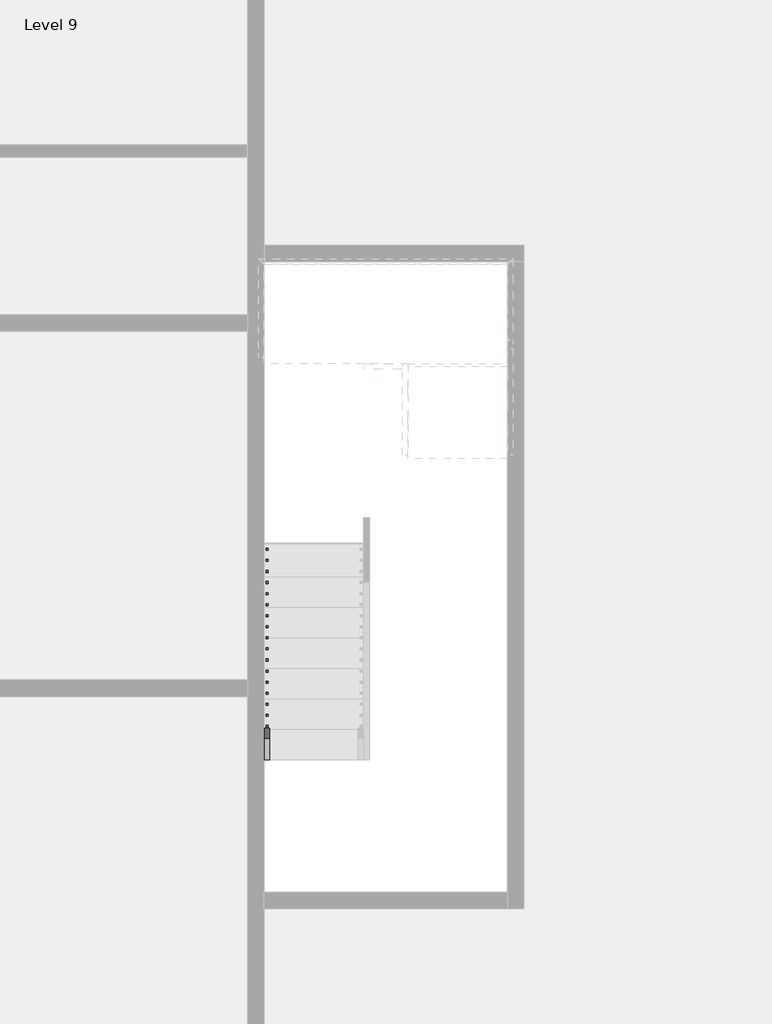
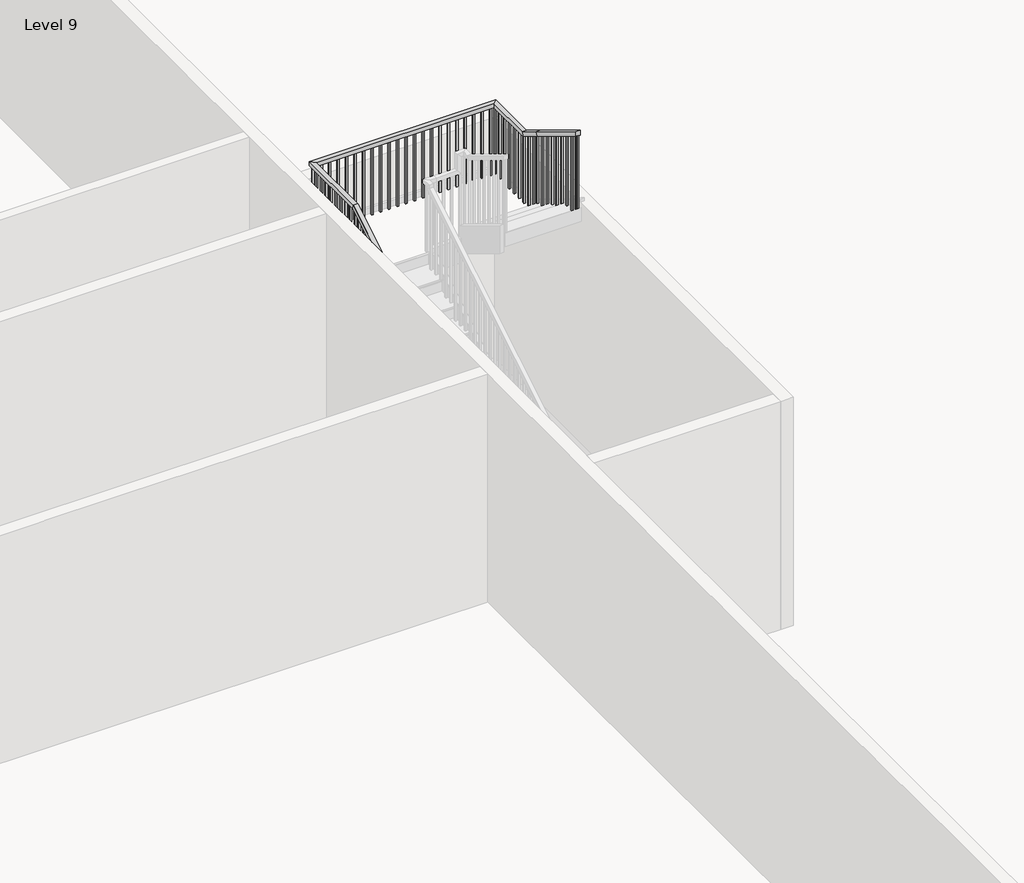
# One storey, part 6 of 8: 1 railing.
"""IFC4 building model written with IfcOpenShell, lengths in millimetres."""

from ifc_helpers import new_model, si_unit, frame, origin, place, context, project, spatial, polyline, outline, extrude, faceted_brep, element, save

model = new_model("IFC4")

# Units and contexts
model_context = context("Model", 3, world=origin())
ifc_project = project(units=[si_unit("LENGTHUNIT", "METRE", prefix="MILLI")], contexts=[model_context])

# Site, building, storey
site = spatial("IfcSite", under=ifc_project)
building = spatial("IfcBuilding", under=site)
storey = spatial("IfcBuildingStorey", under=building, Name="Level 9", Elevation=49618.6172466)

# Railing
placement = place(None, origin())
element("IfcRailing", 1, ObjectType="Handrail - Rectangular", at=placement, inside=storey, context=model_context, shape_type="SolidModel", body=[
    faceted_brep([(-3617.4415084, -23154.3851539, 50702.3505799), (-3617.4415084, -23154.3851539, 50642.9491197), (-3566.6415084, -23154.3851539, 50642.9491197), (-3566.6415084, -23154.3851539, 50702.3505799), (-3617.4415084, -19522.1851539, 52903.6839133), (-3617.4415084, -19507.9927445, 52852.8839133), (-3566.6415084, -19507.9927445, 52852.8839133), (-3566.6415084, -19522.1851539, 52903.6839133), (-3617.4415084, -18607.7851539, 52903.6839133), (-3617.4415084, -18607.7851539, 52852.8839133), (-3566.6415084, -18658.5851539, 52852.8839133), (-3566.6415084, -18658.5851539, 52903.6839133), (-1382.2415084, -18607.7851539, 52903.6839133), (-1382.2415084, -18607.7851539, 52852.8839133), (-1433.0415084, -18658.5851539, 52852.8839133), (-1433.0415084, -18658.5851539, 52903.6839133), (-1382.2415084, -19242.7851539, 52903.6839133), (-1382.2415084, -19256.9775633, 52852.8839133), (-1433.0415084, -19256.9775633, 52852.8839133), (-1433.0415084, -19242.7851539, 52903.6839133), (-1382.2415084, -19522.1851539, 53073.0172466), (-1382.2415084, -19548.5148811, 53029.5731968), (-1433.0415084, -19548.5148811, 53029.5731968), (-1433.0415084, -19522.1851539, 53073.0172466), (-1382.2415084, -20360.3851539, 53581.0172466), (-1433.0415084, -20360.3851539, 53581.0172466), (-1433.0415084, -20360.3851539, 53521.6157863), (-1382.2415084, -20360.3851539, 53521.6157863)], [[[0, 1, 2, 3]], [[1, 0, 4, 5]], [[2, 1, 5, 6]], [[3, 2, 6, 7]], [[0, 3, 7, 4]], [[5, 4, 8, 9]], [[6, 5, 9, 10]], [[7, 6, 10, 11]], [[4, 7, 11, 8]], [[9, 8, 12, 13]], [[10, 9, 13, 14]], [[11, 10, 14, 15]], [[8, 11, 15, 12]], [[13, 12, 16, 17]], [[14, 13, 17, 18]], [[15, 14, 18, 19]], [[12, 15, 19, 16]], [[17, 16, 20, 21]], [[18, 17, 21, 22]], [[19, 18, 22, 23]], [[16, 19, 23, 20]], [[24, 25, 26, 27]], [[21, 20, 24, 27]], [[22, 21, 27, 26]], [[23, 22, 26, 25]], [[20, 23, 25, 24]]]),
    extrude(outline(polyline([(-20325.4601539, 53500.4491197), (-20325.4601539, 52497.2839133), (-20344.5101539, 52497.2839133), (-20344.5101539, 53511.9945742), (-20325.4601539, 53500.4491197)])), frame((-1417.1665084, 0.0, 0.0), z_axis=(1.0, 0.0, 0.0), x_axis=(0.0, 1.0, 0.0)), (0.0, 0.0, 1.0), 19.05),
    extrude(outline(polyline([(-20223.8601539, 53438.8733621), (-20223.8601539, 52497.2839133), (-20242.9101539, 52497.2839133), (-20242.9101539, 53450.4188166), (-20223.8601539, 53438.8733621)])), frame((-1417.1665084, 0.0, 0.0), z_axis=(1.0, 0.0, 0.0), x_axis=(0.0, 1.0, 0.0)), (0.0, 0.0, 1.0), 19.05),
    extrude(outline(polyline([(-20122.2601539, 53377.2976045), (-20122.2601539, 52497.2839133), (-20141.3101539, 52497.2839133), (-20141.3101539, 53388.8430591), (-20122.2601539, 53377.2976045)])), frame((-1417.1665084, 0.0, 0.0), z_axis=(1.0, 0.0, 0.0), x_axis=(0.0, 1.0, 0.0)), (0.0, 0.0, 1.0), 19.05),
    extrude(outline(polyline([(-20020.6601539, 53315.721847), (-20020.6601539, 52327.9505799), (-20039.7101539, 52327.9505799), (-20039.7101539, 53327.2673015), (-20020.6601539, 53315.721847)])), frame((-1417.1665084, 0.0, 0.0), z_axis=(1.0, 0.0, 0.0), x_axis=(0.0, 1.0, 0.0)), (0.0, 0.0, 1.0), 19.05),
    extrude(outline(polyline([(-19919.0601539, 53254.1460894), (-19919.0601539, 52327.9505799), (-19938.1101539, 52327.9505799), (-19938.1101539, 53265.6915439), (-19919.0601539, 53254.1460894)])), frame((-1417.1665084, 0.0, 0.0), z_axis=(1.0, 0.0, 0.0), x_axis=(0.0, 1.0, 0.0)), (0.0, 0.0, 1.0), 19.05),
    extrude(outline(polyline([(-19817.4601539, 53192.5703318), (-19817.4601539, 52327.9505799), (-19836.5101539, 52327.9505799), (-19836.5101539, 53204.1157863), (-19817.4601539, 53192.5703318)])), frame((-1417.1665084, 0.0, 0.0), z_axis=(1.0, 0.0, 0.0), x_axis=(0.0, 1.0, 0.0)), (0.0, 0.0, 1.0), 19.05),
    extrude(outline(polyline([(-19715.8601539, 53130.9945742), (-19715.8601539, 52158.6172466), (-19734.9101539, 52158.6172466), (-19734.9101539, 53142.5400288), (-19715.8601539, 53130.9945742)])), frame((-1417.1665084, 0.0, 0.0), z_axis=(1.0, 0.0, 0.0), x_axis=(0.0, 1.0, 0.0)), (0.0, 0.0, 1.0), 19.05),
    extrude(outline(polyline([(-19614.2601539, 53069.4188166), (-19614.2601539, 52158.6172466), (-19633.3101539, 52158.6172466), (-19633.3101539, 53080.9642712), (-19614.2601539, 53069.4188166)])), frame((-1417.1665084, 0.0, 0.0), z_axis=(1.0, 0.0, 0.0), x_axis=(0.0, 1.0, 0.0)), (0.0, 0.0, 1.0), 19.05),
    extrude(outline(polyline([(-19436.4601539, 52961.6612409), (-19436.4601539, 51989.2839133), (-19455.5101539, 51989.2839133), (-19455.5101539, 52973.2066954), (-19436.4601539, 52961.6612409)])), frame((-1417.1665084, 0.0, 0.0), z_axis=(1.0, 0.0, 0.0), x_axis=(0.0, 1.0, 0.0)), (0.0, 0.0, 1.0), 19.05),
    extrude(outline(polyline([(-19334.8601539, 52900.0854833), (-19334.8601539, 51989.2839133), (-19353.9101539, 51989.2839133), (-19353.9101539, 52911.6309379), (-19334.8601539, 52900.0854833)])), frame((-1417.1665084, 0.0, 0.0), z_axis=(1.0, 0.0, 0.0), x_axis=(0.0, 1.0, 0.0)), (0.0, 0.0, 1.0), 19.05),
    extrude(outline(polyline([(-1398.1165084, -19233.2601539), (-1398.1165084, -19252.3101539), (-1417.1665084, -19252.3101539), (-1417.1665084, -19233.2601539), (-1398.1165084, -19233.2601539)])), frame((0.0, 0.0, 51989.2839133), z_axis=(0.0, 0.0, 1.0), x_axis=(1.0, 0.0, 0.0)), (0.0, 0.0, 1.0), 863.6),
    extrude(outline(polyline([(-1398.1165084, -19131.6601539), (-1398.1165084, -19150.7101539), (-1417.1665084, -19150.7101539), (-1417.1665084, -19131.6601539), (-1398.1165084, -19131.6601539)])), frame((0.0, 0.0, 51989.2839133), z_axis=(0.0, 0.0, 1.0), x_axis=(1.0, 0.0, 0.0)), (0.0, 0.0, 1.0), 863.6),
    extrude(outline(polyline([(-1398.1165084, -19030.0601539), (-1398.1165084, -19049.1101539), (-1417.1665084, -19049.1101539), (-1417.1665084, -19030.0601539), (-1398.1165084, -19030.0601539)])), frame((0.0, 0.0, 51989.2839133), z_axis=(0.0, 0.0, 1.0), x_axis=(1.0, 0.0, 0.0)), (0.0, 0.0, 1.0), 863.6),
    extrude(outline(polyline([(-1398.1165084, -18928.4601539), (-1398.1165084, -18947.5101539), (-1417.1665084, -18947.5101539), (-1417.1665084, -18928.4601539), (-1398.1165084, -18928.4601539)])), frame((0.0, 0.0, 51989.2839133), z_axis=(0.0, 0.0, 1.0), x_axis=(1.0, 0.0, 0.0)), (0.0, 0.0, 1.0), 863.6),
    extrude(outline(polyline([(-1398.1165084, -18826.8601539), (-1398.1165084, -18845.9101539), (-1417.1665084, -18845.9101539), (-1417.1665084, -18826.8601539), (-1398.1165084, -18826.8601539)])), frame((0.0, 0.0, 51989.2839133), z_axis=(0.0, 0.0, 1.0), x_axis=(1.0, 0.0, 0.0)), (0.0, 0.0, 1.0), 863.6),
    extrude(outline(polyline([(-1398.1165084, -18725.2601539), (-1398.1165084, -18744.3101539), (-1417.1665084, -18744.3101539), (-1417.1665084, -18725.2601539), (-1398.1165084, -18725.2601539)])), frame((0.0, 0.0, 51989.2839133), z_axis=(0.0, 0.0, 1.0), x_axis=(1.0, 0.0, 0.0)), (0.0, 0.0, 1.0), 863.6),
    extrude(outline(polyline([(-1467.9665084, -18623.6601539), (-1448.9165084, -18623.6601539), (-1448.9165084, -18642.7101539), (-1467.9665084, -18642.7101539), (-1467.9665084, -18623.6601539)])), frame((0.0, 0.0, 51989.2839133), z_axis=(0.0, 0.0, 1.0), x_axis=(1.0, 0.0, 0.0)), (0.0, 0.0, 1.0), 863.6),
    extrude(outline(polyline([(-1569.5665084, -18623.6601539), (-1550.5165084, -18623.6601539), (-1550.5165084, -18642.7101539), (-1569.5665084, -18642.7101539), (-1569.5665084, -18623.6601539)])), frame((0.0, 0.0, 51989.2839133), z_axis=(0.0, 0.0, 1.0), x_axis=(1.0, 0.0, 0.0)), (0.0, 0.0, 1.0), 863.6),
    extrude(outline(polyline([(-1671.1665084, -18623.6601539), (-1652.1165084, -18623.6601539), (-1652.1165084, -18642.7101539), (-1671.1665084, -18642.7101539), (-1671.1665084, -18623.6601539)])), frame((0.0, 0.0, 51989.2839133), z_axis=(0.0, 0.0, 1.0), x_axis=(1.0, 0.0, 0.0)), (0.0, 0.0, 1.0), 863.6),
    extrude(outline(polyline([(-1772.7665084, -18623.6601539), (-1753.7165084, -18623.6601539), (-1753.7165084, -18642.7101539), (-1772.7665084, -18642.7101539), (-1772.7665084, -18623.6601539)])), frame((0.0, 0.0, 51989.2839133), z_axis=(0.0, 0.0, 1.0), x_axis=(1.0, 0.0, 0.0)), (0.0, 0.0, 1.0), 863.6),
    extrude(outline(polyline([(-1874.3665084, -18623.6601539), (-1855.3165084, -18623.6601539), (-1855.3165084, -18642.7101539), (-1874.3665084, -18642.7101539), (-1874.3665084, -18623.6601539)])), frame((0.0, 0.0, 51989.2839133), z_axis=(0.0, 0.0, 1.0), x_axis=(1.0, 0.0, 0.0)), (0.0, 0.0, 1.0), 863.6),
    extrude(outline(polyline([(-1975.9665084, -18623.6601539), (-1956.9165084, -18623.6601539), (-1956.9165084, -18642.7101539), (-1975.9665084, -18642.7101539), (-1975.9665084, -18623.6601539)])), frame((0.0, 0.0, 51989.2839133), z_axis=(0.0, 0.0, 1.0), x_axis=(1.0, 0.0, 0.0)), (0.0, 0.0, 1.0), 863.6),
    extrude(outline(polyline([(-2077.5665084, -18623.6601539), (-2058.5165084, -18623.6601539), (-2058.5165084, -18642.7101539), (-2077.5665084, -18642.7101539), (-2077.5665084, -18623.6601539)])), frame((0.0, 0.0, 51989.2839133), z_axis=(0.0, 0.0, 1.0), x_axis=(1.0, 0.0, 0.0)), (0.0, 0.0, 1.0), 863.6),
    extrude(outline(polyline([(-2179.1665084, -18623.6601539), (-2160.1165084, -18623.6601539), (-2160.1165084, -18642.7101539), (-2179.1665084, -18642.7101539), (-2179.1665084, -18623.6601539)])), frame((0.0, 0.0, 51989.2839133), z_axis=(0.0, 0.0, 1.0), x_axis=(1.0, 0.0, 0.0)), (0.0, 0.0, 1.0), 863.6),
    extrude(outline(polyline([(-2280.7665084, -18623.6601539), (-2261.7165084, -18623.6601539), (-2261.7165084, -18642.7101539), (-2280.7665084, -18642.7101539), (-2280.7665084, -18623.6601539)])), frame((0.0, 0.0, 51989.2839133), z_axis=(0.0, 0.0, 1.0), x_axis=(1.0, 0.0, 0.0)), (0.0, 0.0, 1.0), 863.6),
    extrude(outline(polyline([(-2382.3665084, -18623.6601539), (-2363.3165084, -18623.6601539), (-2363.3165084, -18642.7101539), (-2382.3665084, -18642.7101539), (-2382.3665084, -18623.6601539)])), frame((0.0, 0.0, 51989.2839133), z_axis=(0.0, 0.0, 1.0), x_axis=(1.0, 0.0, 0.0)), (0.0, 0.0, 1.0), 863.6),
    extrude(outline(polyline([(-2483.9665084, -18623.6601539), (-2464.9165084, -18623.6601539), (-2464.9165084, -18642.7101539), (-2483.9665084, -18642.7101539), (-2483.9665084, -18623.6601539)])), frame((0.0, 0.0, 51989.2839133), z_axis=(0.0, 0.0, 1.0), x_axis=(1.0, 0.0, 0.0)), (0.0, 0.0, 1.0), 863.6),
    extrude(outline(polyline([(-2585.5665084, -18623.6601539), (-2566.5165084, -18623.6601539), (-2566.5165084, -18642.7101539), (-2585.5665084, -18642.7101539), (-2585.5665084, -18623.6601539)])), frame((0.0, 0.0, 51989.2839133), z_axis=(0.0, 0.0, 1.0), x_axis=(1.0, 0.0, 0.0)), (0.0, 0.0, 1.0), 863.6),
    extrude(outline(polyline([(-2687.1665084, -18623.6601539), (-2668.1165084, -18623.6601539), (-2668.1165084, -18642.7101539), (-2687.1665084, -18642.7101539), (-2687.1665084, -18623.6601539)])), frame((0.0, 0.0, 51989.2839133), z_axis=(0.0, 0.0, 1.0), x_axis=(1.0, 0.0, 0.0)), (0.0, 0.0, 1.0), 863.6),
    extrude(outline(polyline([(-2788.7665084, -18623.6601539), (-2769.7165084, -18623.6601539), (-2769.7165084, -18642.7101539), (-2788.7665084, -18642.7101539), (-2788.7665084, -18623.6601539)])), frame((0.0, 0.0, 51989.2839133), z_axis=(0.0, 0.0, 1.0), x_axis=(1.0, 0.0, 0.0)), (0.0, 0.0, 1.0), 863.6),
    extrude(outline(polyline([(-2890.3665084, -18623.6601539), (-2871.3165084, -18623.6601539), (-2871.3165084, -18642.7101539), (-2890.3665084, -18642.7101539), (-2890.3665084, -18623.6601539)])), frame((0.0, 0.0, 51989.2839133), z_axis=(0.0, 0.0, 1.0), x_axis=(1.0, 0.0, 0.0)), (0.0, 0.0, 1.0), 863.6),
    extrude(outline(polyline([(-2991.9665084, -18623.6601539), (-2972.9165084, -18623.6601539), (-2972.9165084, -18642.7101539), (-2991.9665084, -18642.7101539), (-2991.9665084, -18623.6601539)])), frame((0.0, 0.0, 51989.2839133), z_axis=(0.0, 0.0, 1.0), x_axis=(1.0, 0.0, 0.0)), (0.0, 0.0, 1.0), 863.6),
    extrude(outline(polyline([(-3093.5665084, -18623.6601539), (-3074.5165084, -18623.6601539), (-3074.5165084, -18642.7101539), (-3093.5665084, -18642.7101539), (-3093.5665084, -18623.6601539)])), frame((0.0, 0.0, 51989.2839133), z_axis=(0.0, 0.0, 1.0), x_axis=(1.0, 0.0, 0.0)), (0.0, 0.0, 1.0), 863.6),
    extrude(outline(polyline([(-3195.1665084, -18623.6601539), (-3176.1165084, -18623.6601539), (-3176.1165084, -18642.7101539), (-3195.1665084, -18642.7101539), (-3195.1665084, -18623.6601539)])), frame((0.0, 0.0, 51989.2839133), z_axis=(0.0, 0.0, 1.0), x_axis=(1.0, 0.0, 0.0)), (0.0, 0.0, 1.0), 863.6),
    extrude(outline(polyline([(-3296.7665084, -18623.6601539), (-3277.7165084, -18623.6601539), (-3277.7165084, -18642.7101539), (-3296.7665084, -18642.7101539), (-3296.7665084, -18623.6601539)])), frame((0.0, 0.0, 51989.2839133), z_axis=(0.0, 0.0, 1.0), x_axis=(1.0, 0.0, 0.0)), (0.0, 0.0, 1.0), 863.6),
    extrude(outline(polyline([(-3398.3665084, -18623.6601539), (-3379.3165084, -18623.6601539), (-3379.3165084, -18642.7101539), (-3398.3665084, -18642.7101539), (-3398.3665084, -18623.6601539)])), frame((0.0, 0.0, 51989.2839133), z_axis=(0.0, 0.0, 1.0), x_axis=(1.0, 0.0, 0.0)), (0.0, 0.0, 1.0), 863.6),
    extrude(outline(polyline([(-3499.9665084, -18623.6601539), (-3480.9165084, -18623.6601539), (-3480.9165084, -18642.7101539), (-3499.9665084, -18642.7101539), (-3499.9665084, -18623.6601539)])), frame((0.0, 0.0, 51989.2839133), z_axis=(0.0, 0.0, 1.0), x_axis=(1.0, 0.0, 0.0)), (0.0, 0.0, 1.0), 863.6),
    extrude(outline(polyline([(-3601.5665084, -18718.9101539), (-3601.5665084, -18699.8601539), (-3582.5165084, -18699.8601539), (-3582.5165084, -18718.9101539), (-3601.5665084, -18718.9101539)])), frame((0.0, 0.0, 51989.2839133), z_axis=(0.0, 0.0, 1.0), x_axis=(1.0, 0.0, 0.0)), (0.0, 0.0, 1.0), 863.6),
    extrude(outline(polyline([(-3601.5665084, -18820.5101539), (-3601.5665084, -18801.4601539), (-3582.5165084, -18801.4601539), (-3582.5165084, -18820.5101539), (-3601.5665084, -18820.5101539)])), frame((0.0, 0.0, 51989.2839133), z_axis=(0.0, 0.0, 1.0), x_axis=(1.0, 0.0, 0.0)), (0.0, 0.0, 1.0), 863.6),
    extrude(outline(polyline([(-3601.5665084, -18922.1101539), (-3601.5665084, -18903.0601539), (-3582.5165084, -18903.0601539), (-3582.5165084, -18922.1101539), (-3601.5665084, -18922.1101539)])), frame((0.0, 0.0, 51989.2839133), z_axis=(0.0, 0.0, 1.0), x_axis=(1.0, 0.0, 0.0)), (0.0, 0.0, 1.0), 863.6),
    extrude(outline(polyline([(-3601.5665084, -19023.7101539), (-3601.5665084, -19004.6601539), (-3582.5165084, -19004.6601539), (-3582.5165084, -19023.7101539), (-3601.5665084, -19023.7101539)])), frame((0.0, 0.0, 51989.2839133), z_axis=(0.0, 0.0, 1.0), x_axis=(1.0, 0.0, 0.0)), (0.0, 0.0, 1.0), 863.6),
    extrude(outline(polyline([(-3601.5665084, -19125.3101539), (-3601.5665084, -19106.2601539), (-3582.5165084, -19106.2601539), (-3582.5165084, -19125.3101539), (-3601.5665084, -19125.3101539)])), frame((0.0, 0.0, 51989.2839133), z_axis=(0.0, 0.0, 1.0), x_axis=(1.0, 0.0, 0.0)), (0.0, 0.0, 1.0), 863.6),
    extrude(outline(polyline([(-3601.5665084, -19226.9101539), (-3601.5665084, -19207.8601539), (-3582.5165084, -19207.8601539), (-3582.5165084, -19226.9101539), (-3601.5665084, -19226.9101539)])), frame((0.0, 0.0, 51989.2839133), z_axis=(0.0, 0.0, 1.0), x_axis=(1.0, 0.0, 0.0)), (0.0, 0.0, 1.0), 863.6),
    extrude(outline(polyline([(-3601.5665084, -19328.5101539), (-3601.5665084, -19309.4601539), (-3582.5165084, -19309.4601539), (-3582.5165084, -19328.5101539), (-3601.5665084, -19328.5101539)])), frame((0.0, 0.0, 51989.2839133), z_axis=(0.0, 0.0, 1.0), x_axis=(1.0, 0.0, 0.0)), (0.0, 0.0, 1.0), 863.6),
    extrude(outline(polyline([(-3601.5665084, -19430.1101539), (-3601.5665084, -19411.0601539), (-3582.5165084, -19411.0601539), (-3582.5165084, -19430.1101539), (-3601.5665084, -19430.1101539)])), frame((0.0, 0.0, 51989.2839133), z_axis=(0.0, 0.0, 1.0), x_axis=(1.0, 0.0, 0.0)), (0.0, 0.0, 1.0), 863.6),
    extrude(outline(polyline([(-19588.8601539, 52803.8733621), (-19588.8601539, 51819.9505799), (-19607.9101539, 51819.9505799), (-19607.9101539, 52792.3279076), (-19588.8601539, 52803.8733621)])), frame((-3601.5665084, 0.0, 0.0), z_axis=(1.0, 0.0, 0.0), x_axis=(0.0, 1.0, 0.0)), (0.0, 0.0, 1.0), 19.05),
    extrude(outline(polyline([(-19690.4601539, 52742.2976045), (-19690.4601539, 51819.9505799), (-19709.5101539, 51819.9505799), (-19709.5101539, 52730.75215), (-19690.4601539, 52742.2976045)])), frame((-3601.5665084, 0.0, 0.0), z_axis=(1.0, 0.0, 0.0), x_axis=(0.0, 1.0, 0.0)), (0.0, 0.0, 1.0), 19.05),
    extrude(outline(polyline([(-19792.0601539, 52680.721847), (-19792.0601539, 51819.9505799), (-19811.1101539, 51819.9505799), (-19811.1101539, 52669.1763924), (-19792.0601539, 52680.721847)])), frame((-3601.5665084, 0.0, 0.0), z_axis=(1.0, 0.0, 0.0), x_axis=(0.0, 1.0, 0.0)), (0.0, 0.0, 1.0), 19.05),
    extrude(outline(polyline([(-19893.6601539, 52619.1460894), (-19893.6601539, 51650.6172466), (-19912.7101539, 51650.6172466), (-19912.7101539, 52607.6006348), (-19893.6601539, 52619.1460894)])), frame((-3601.5665084, 0.0, 0.0), z_axis=(1.0, 0.0, 0.0), x_axis=(0.0, 1.0, 0.0)), (0.0, 0.0, 1.0), 19.05),
    extrude(outline(polyline([(-19995.2601539, 52557.5703318), (-19995.2601539, 51650.6172466), (-20014.3101539, 51650.6172466), (-20014.3101539, 52546.0248773), (-19995.2601539, 52557.5703318)])), frame((-3601.5665084, 0.0, 0.0), z_axis=(1.0, 0.0, 0.0), x_axis=(0.0, 1.0, 0.0)), (0.0, 0.0, 1.0), 19.05),
    extrude(outline(polyline([(-20096.8601539, 52495.9945742), (-20096.8601539, 51481.2839133), (-20115.9101539, 51481.2839133), (-20115.9101539, 52484.4491197), (-20096.8601539, 52495.9945742)])), frame((-3601.5665084, 0.0, 0.0), z_axis=(1.0, 0.0, 0.0), x_axis=(0.0, 1.0, 0.0)), (0.0, 0.0, 1.0), 19.05),
    extrude(outline(polyline([(-20198.4601539, 52434.4188166), (-20198.4601539, 51481.2839133), (-20217.5101539, 51481.2839133), (-20217.5101539, 52422.8733621), (-20198.4601539, 52434.4188166)])), frame((-3601.5665084, 0.0, 0.0), z_axis=(1.0, 0.0, 0.0), x_axis=(0.0, 1.0, 0.0)), (0.0, 0.0, 1.0), 19.05),
    extrude(outline(polyline([(-20300.0601539, 52372.8430591), (-20300.0601539, 51481.2839133), (-20319.1101539, 51481.2839133), (-20319.1101539, 52361.2976045), (-20300.0601539, 52372.8430591)])), frame((-3601.5665084, 0.0, 0.0), z_axis=(1.0, 0.0, 0.0), x_axis=(0.0, 1.0, 0.0)), (0.0, 0.0, 1.0), 19.05),
    extrude(outline(polyline([(-20401.6601539, 52311.2673015), (-20401.6601539, 51311.9505799), (-20420.7101539, 51311.9505799), (-20420.7101539, 52299.721847), (-20401.6601539, 52311.2673015)])), frame((-3601.5665084, 0.0, 0.0), z_axis=(1.0, 0.0, 0.0), x_axis=(0.0, 1.0, 0.0)), (0.0, 0.0, 1.0), 19.05),
    extrude(outline(polyline([(-20503.2601539, 52249.6915439), (-20503.2601539, 51311.9505799), (-20522.3101539, 51311.9505799), (-20522.3101539, 52238.1460894), (-20503.2601539, 52249.6915439)])), frame((-3601.5665084, 0.0, 0.0), z_axis=(1.0, 0.0, 0.0), x_axis=(0.0, 1.0, 0.0)), (0.0, 0.0, 1.0), 19.05),
    extrude(outline(polyline([(-20604.8601539, 52188.1157863), (-20604.8601539, 51311.9505799), (-20623.9101539, 51311.9505799), (-20623.9101539, 52176.5703318), (-20604.8601539, 52188.1157863)])), frame((-3601.5665084, 0.0, 0.0), z_axis=(1.0, 0.0, 0.0), x_axis=(0.0, 1.0, 0.0)), (0.0, 0.0, 1.0), 19.05),
    extrude(outline(polyline([(-20706.4601539, 52126.5400288), (-20706.4601539, 51142.6172466), (-20725.5101539, 51142.6172466), (-20725.5101539, 52114.9945742), (-20706.4601539, 52126.5400288)])), frame((-3601.5665084, 0.0, 0.0), z_axis=(1.0, 0.0, 0.0), x_axis=(0.0, 1.0, 0.0)), (0.0, 0.0, 1.0), 19.05),
    extrude(outline(polyline([(-20808.0601539, 52064.9642712), (-20808.0601539, 51142.6172466), (-20827.1101539, 51142.6172466), (-20827.1101539, 52053.4188166), (-20808.0601539, 52064.9642712)])), frame((-3601.5665084, 0.0, 0.0), z_axis=(1.0, 0.0, 0.0), x_axis=(0.0, 1.0, 0.0)), (0.0, 0.0, 1.0), 19.05),
    extrude(outline(polyline([(-20909.6601539, 52003.3885136), (-20909.6601539, 51142.6172466), (-20928.7101539, 51142.6172466), (-20928.7101539, 51991.8430591), (-20909.6601539, 52003.3885136)])), frame((-3601.5665084, 0.0, 0.0), z_axis=(1.0, 0.0, 0.0), x_axis=(0.0, 1.0, 0.0)), (0.0, 0.0, 1.0), 19.05),
    extrude(outline(polyline([(-21011.2601539, 51941.812756), (-21011.2601539, 50973.2839133), (-21030.3101539, 50973.2839133), (-21030.3101539, 51930.2673015), (-21011.2601539, 51941.812756)])), frame((-3601.5665084, 0.0, 0.0), z_axis=(1.0, 0.0, 0.0), x_axis=(0.0, 1.0, 0.0)), (0.0, 0.0, 1.0), 19.05),
    extrude(outline(polyline([(-21112.8601539, 51880.2369985), (-21112.8601539, 50973.2839133), (-21131.9101539, 50973.2839133), (-21131.9101539, 51868.6915439), (-21112.8601539, 51880.2369985)])), frame((-3601.5665084, 0.0, 0.0), z_axis=(1.0, 0.0, 0.0), x_axis=(0.0, 1.0, 0.0)), (0.0, 0.0, 1.0), 19.05),
    extrude(outline(polyline([(-21214.4601539, 51818.6612409), (-21214.4601539, 50803.9505799), (-21233.5101539, 50803.9505799), (-21233.5101539, 51807.1157863), (-21214.4601539, 51818.6612409)])), frame((-3601.5665084, 0.0, 0.0), z_axis=(1.0, 0.0, 0.0), x_axis=(0.0, 1.0, 0.0)), (0.0, 0.0, 1.0), 19.05),
    extrude(outline(polyline([(-21316.0601539, 51757.0854833), (-21316.0601539, 50803.9505799), (-21335.1101539, 50803.9505799), (-21335.1101539, 51745.5400288), (-21316.0601539, 51757.0854833)])), frame((-3601.5665084, 0.0, 0.0), z_axis=(1.0, 0.0, 0.0), x_axis=(0.0, 1.0, 0.0)), (0.0, 0.0, 1.0), 19.05),
    extrude(outline(polyline([(-21417.6601539, 51695.5097257), (-21417.6601539, 50803.9505799), (-21436.7101539, 50803.9505799), (-21436.7101539, 51683.9642712), (-21417.6601539, 51695.5097257)])), frame((-3601.5665084, 0.0, 0.0), z_axis=(1.0, 0.0, 0.0), x_axis=(0.0, 1.0, 0.0)), (0.0, 0.0, 1.0), 19.05),
    extrude(outline(polyline([(-21519.2601539, 51633.9339682), (-21519.2601539, 50634.6172466), (-21538.3101539, 50634.6172466), (-21538.3101539, 51622.3885136), (-21519.2601539, 51633.9339682)])), frame((-3601.5665084, 0.0, 0.0), z_axis=(1.0, 0.0, 0.0), x_axis=(0.0, 1.0, 0.0)), (0.0, 0.0, 1.0), 19.05),
    extrude(outline(polyline([(-21620.8601539, 51572.3582106), (-21620.8601539, 50634.6172466), (-21639.9101539, 50634.6172466), (-21639.9101539, 51560.812756), (-21620.8601539, 51572.3582106)])), frame((-3601.5665084, 0.0, 0.0), z_axis=(1.0, 0.0, 0.0), x_axis=(0.0, 1.0, 0.0)), (0.0, 0.0, 1.0), 19.05),
    extrude(outline(polyline([(-21722.4601539, 51510.782453), (-21722.4601539, 50634.6172466), (-21741.5101539, 50634.6172466), (-21741.5101539, 51499.2369985), (-21722.4601539, 51510.782453)])), frame((-3601.5665084, 0.0, 0.0), z_axis=(1.0, 0.0, 0.0), x_axis=(0.0, 1.0, 0.0)), (0.0, 0.0, 1.0), 19.05),
    extrude(outline(polyline([(-21824.0601539, 51449.2066954), (-21824.0601539, 50465.2839133), (-21843.1101539, 50465.2839133), (-21843.1101539, 51437.6612409), (-21824.0601539, 51449.2066954)])), frame((-3601.5665084, 0.0, 0.0), z_axis=(1.0, 0.0, 0.0), x_axis=(0.0, 1.0, 0.0)), (0.0, 0.0, 1.0), 19.05),
    extrude(outline(polyline([(-21925.6601539, 51387.6309379), (-21925.6601539, 50465.2839133), (-21944.7101539, 50465.2839133), (-21944.7101539, 51376.0854833), (-21925.6601539, 51387.6309379)])), frame((-3601.5665084, 0.0, 0.0), z_axis=(1.0, 0.0, 0.0), x_axis=(0.0, 1.0, 0.0)), (0.0, 0.0, 1.0), 19.05),
    extrude(outline(polyline([(-22027.2601539, 51326.0551803), (-22027.2601539, 50465.2839133), (-22046.3101539, 50465.2839133), (-22046.3101539, 51314.5097257), (-22027.2601539, 51326.0551803)])), frame((-3601.5665084, 0.0, 0.0), z_axis=(1.0, 0.0, 0.0), x_axis=(0.0, 1.0, 0.0)), (0.0, 0.0, 1.0), 19.05),
    extrude(outline(polyline([(-22128.8601539, 51264.4794227), (-22128.8601539, 50295.9505799), (-22147.9101539, 50295.9505799), (-22147.9101539, 51252.9339682), (-22128.8601539, 51264.4794227)])), frame((-3601.5665084, 0.0, 0.0), z_axis=(1.0, 0.0, 0.0), x_axis=(0.0, 1.0, 0.0)), (0.0, 0.0, 1.0), 19.05),
    extrude(outline(polyline([(-22230.4601539, 51202.9036651), (-22230.4601539, 50295.9505799), (-22249.5101539, 50295.9505799), (-22249.5101539, 51191.3582106), (-22230.4601539, 51202.9036651)])), frame((-3601.5665084, 0.0, 0.0), z_axis=(1.0, 0.0, 0.0), x_axis=(0.0, 1.0, 0.0)), (0.0, 0.0, 1.0), 19.05),
    extrude(outline(polyline([(-22332.0601539, 51141.3279076), (-22332.0601539, 50126.6172466), (-22351.1101539, 50126.6172466), (-22351.1101539, 51129.782453), (-22332.0601539, 51141.3279076)])), frame((-3601.5665084, 0.0, 0.0), z_axis=(1.0, 0.0, 0.0), x_axis=(0.0, 1.0, 0.0)), (0.0, 0.0, 1.0), 19.05),
    extrude(outline(polyline([(-22433.6601539, 51079.75215), (-22433.6601539, 50126.6172466), (-22452.7101539, 50126.6172466), (-22452.7101539, 51068.2066954), (-22433.6601539, 51079.75215)])), frame((-3601.5665084, 0.0, 0.0), z_axis=(1.0, 0.0, 0.0), x_axis=(0.0, 1.0, 0.0)), (0.0, 0.0, 1.0), 19.05),
    extrude(outline(polyline([(-22535.2601539, 51018.1763924), (-22535.2601539, 50126.6172466), (-22554.3101539, 50126.6172466), (-22554.3101539, 51006.6309379), (-22535.2601539, 51018.1763924)])), frame((-3601.5665084, 0.0, 0.0), z_axis=(1.0, 0.0, 0.0), x_axis=(0.0, 1.0, 0.0)), (0.0, 0.0, 1.0), 19.05),
    extrude(outline(polyline([(-22636.8601539, 50956.6006348), (-22636.8601539, 49957.2839133), (-22655.9101539, 49957.2839133), (-22655.9101539, 50945.0551803), (-22636.8601539, 50956.6006348)])), frame((-3601.5665084, 0.0, 0.0), z_axis=(1.0, 0.0, 0.0), x_axis=(0.0, 1.0, 0.0)), (0.0, 0.0, 1.0), 19.05),
    extrude(outline(polyline([(-22738.4601539, 50895.0248773), (-22738.4601539, 49957.2839133), (-22757.5101539, 49957.2839133), (-22757.5101539, 50883.4794227), (-22738.4601539, 50895.0248773)])), frame((-3601.5665084, 0.0, 0.0), z_axis=(1.0, 0.0, 0.0), x_axis=(0.0, 1.0, 0.0)), (0.0, 0.0, 1.0), 19.05),
    extrude(outline(polyline([(-22840.0601539, 50833.4491197), (-22840.0601539, 49957.2839133), (-22859.1101539, 49957.2839133), (-22859.1101539, 50821.9036651), (-22840.0601539, 50833.4491197)])), frame((-3601.5665084, 0.0, 0.0), z_axis=(1.0, 0.0, 0.0), x_axis=(0.0, 1.0, 0.0)), (0.0, 0.0, 1.0), 19.05),
    extrude(outline(polyline([(-22941.6601539, 50771.8733621), (-22941.6601539, 49787.9505799), (-22960.7101539, 49787.9505799), (-22960.7101539, 50760.3279076), (-22941.6601539, 50771.8733621)])), frame((-3601.5665084, 0.0, 0.0), z_axis=(1.0, 0.0, 0.0), x_axis=(0.0, 1.0, 0.0)), (0.0, 0.0, 1.0), 19.05),
    extrude(outline(polyline([(-23043.2601539, 50710.2976045), (-23043.2601539, 49787.9505799), (-23062.3101539, 49787.9505799), (-23062.3101539, 50698.75215), (-23043.2601539, 50710.2976045)])), frame((-3601.5665084, 0.0, 0.0), z_axis=(1.0, 0.0, 0.0), x_axis=(0.0, 1.0, 0.0)), (0.0, 0.0, 1.0), 19.05),
    extrude(outline(polyline([(-19512.6601539, 53007.8430591), (-19512.6601539, 51989.2839133), (-19531.7101539, 51989.2839133), (-19531.7101539, 53019.3885136), (-19512.6601539, 53007.8430591)])), frame((-1417.1665084, 0.0, 0.0), z_axis=(1.0, 0.0, 0.0), x_axis=(0.0, 1.0, 0.0)), (0.0, 0.0, 1.0), 19.05),
    extrude(outline(polyline([(-1417.1665084, -18623.6601539), (-1398.1165084, -18623.6601539), (-1398.1165084, -18642.7101539), (-1417.1665084, -18642.7101539), (-1417.1665084, -18623.6601539)])), frame((0.0, 0.0, 51989.2839133), z_axis=(0.0, 0.0, 1.0), x_axis=(1.0, 0.0, 0.0)), (0.0, 0.0, 1.0), 863.6),
    extrude(outline(polyline([(-3601.5665084, -18642.7101539), (-3601.5665084, -18623.6601539), (-3582.5165084, -18623.6601539), (-3582.5165084, -18642.7101539), (-3601.5665084, -18642.7101539)])), frame((0.0, 0.0, 51989.2839133), z_axis=(0.0, 0.0, 1.0), x_axis=(1.0, 0.0, 0.0)), (0.0, 0.0, 1.0), 863.6),
    extrude(outline(polyline([(-19512.6601539, 52850.0551803), (-19512.6601539, 51989.2839133), (-19531.7101539, 51989.2839133), (-19531.7101539, 52838.5097257), (-19512.6601539, 52850.0551803)])), frame((-3601.5665084, 0.0, 0.0), z_axis=(1.0, 0.0, 0.0), x_axis=(0.0, 1.0, 0.0)), (0.0, 0.0, 1.0), 19.05),
    extrude(outline(polyline([(-20341.3351539, 53510.0703318), (-20341.3351539, 52497.2839133), (-20360.3851539, 52497.2839133), (-20360.3851539, 53521.6157863), (-20341.3351539, 53510.0703318)])), frame((-1417.1665084, 0.0, 0.0), z_axis=(1.0, 0.0, 0.0), x_axis=(0.0, 1.0, 0.0)), (0.0, 0.0, 1.0), 19.05),
    extrude(outline(polyline([(-23135.3351539, 50654.4945742), (-23135.3351539, 49787.9505799), (-23154.3851539, 49787.9505799), (-23154.3851539, 50642.9491197), (-23135.3351539, 50654.4945742)])), frame((-3601.5665084, 0.0, 0.0), z_axis=(1.0, 0.0, 0.0), x_axis=(0.0, 1.0, 0.0)), (0.0, 0.0, 1.0), 19.05),
])

save(model, "model.ifc")

# Revit data of these elements
# Type "Handrail - Rectangular"
#   Assembly Code = "C2010400"
#   built-in parameter 1008612 = 0.0416667 (stored number, unit not read)
#   built-in parameter 1008611 = 0.0416667 (stored number, unit not read)
#   built-in parameter 1008609 = 0.333333 (stored number, unit not read)
#   built-in parameter 1008604 = 0.166667 (stored number, unit not read)
#   built-in parameter 1008603 = 0.166667 (stored number, unit not read)
#   Railing Height = 3' - 0"
#   built-in parameter 1008630 = 2
#   built-in parameter 1008610 = 2
#   built-in parameter 1008618 = Baluster - Square : 3/4"
# Element 1 (IfcRailing, "Handrail - Rectangular")
#   Phase Created = New Construction
